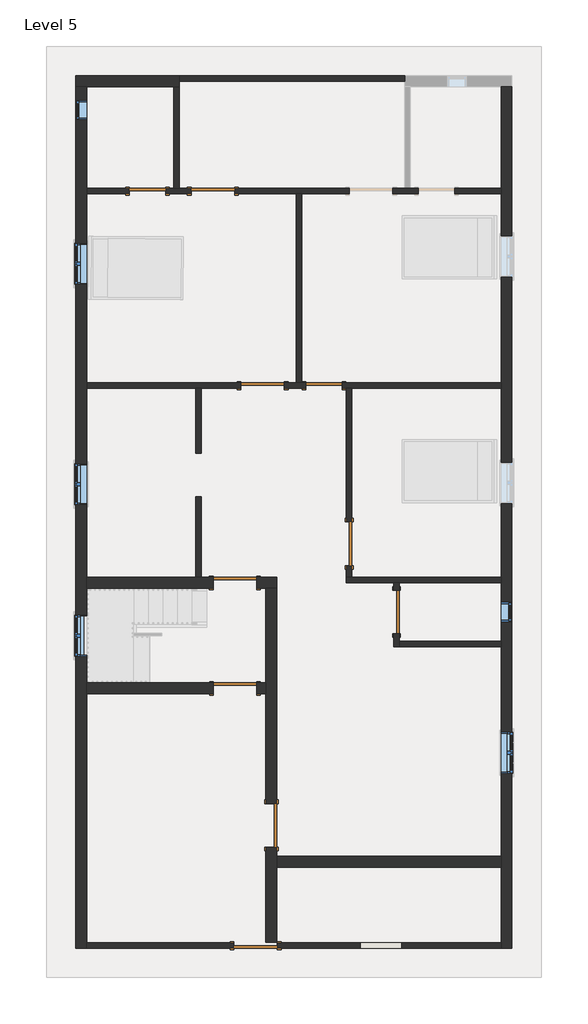
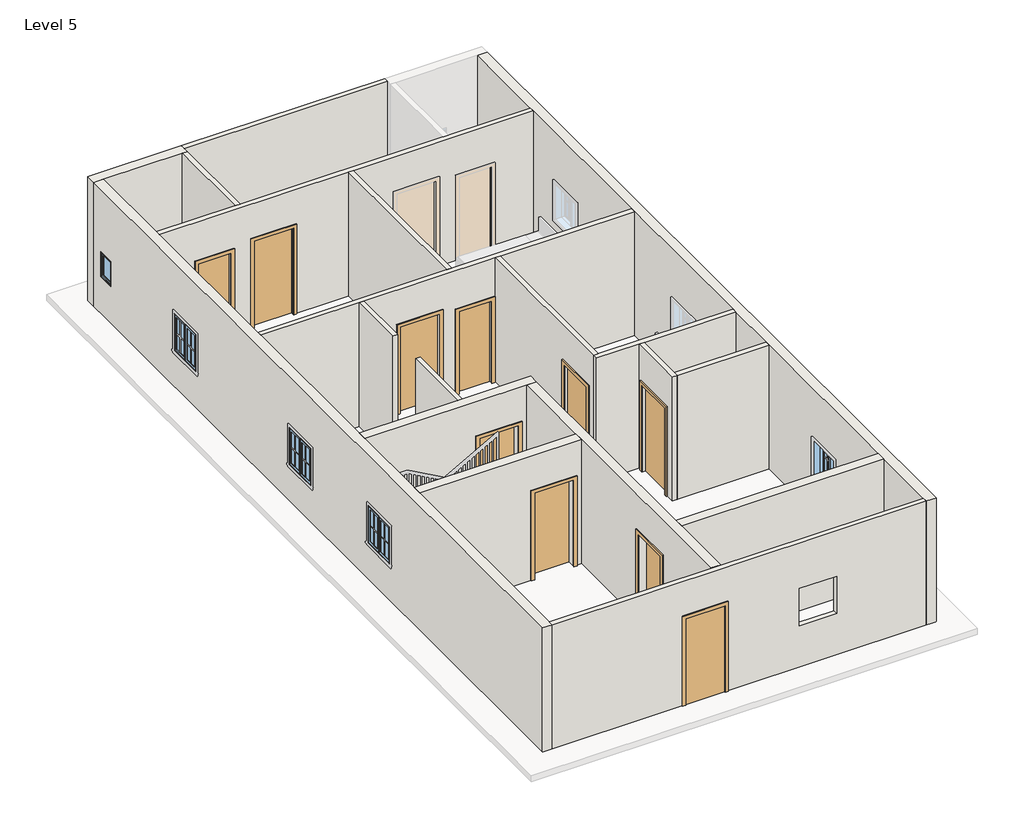
# One storey, part 1 of 3: 19 walls, 10 doors, 6 windows.
"""IFC4 building model written with IfcOpenShell, lengths in millimetres."""

from ifc_helpers import new_model, si_unit, frame, origin, place, context, project, spatial, polyline, outline, extrude, faceted_brep, transform, mapped, element, save
from components import door_d8f5dbb5, door_f2b275c1, door_e5f9f3c4, door_0ca8825f, door_305aa2a5, window_aa618e30, window_339605e1

model = new_model("IFC4")

# Units and contexts
model_context = context("Model", 3, world=origin())
ifc_project = project(units=[si_unit("LENGTHUNIT", "METRE", prefix="MILLI")], contexts=[model_context])

# Site, building, storey
site = spatial("IfcSite", under=ifc_project)
building = spatial("IfcBuilding", under=site)
storey = spatial("IfcBuildingStorey", under=building, Name="Level 5", Elevation=9601.2)

# Doors
placement = place(None, origin())
door_shape = door_d8f5dbb5(model_context)
element("IfcDoor", 1, ObjectType="Single-Flush : 30\" x 80\"", at=placement, inside=storey, context=model_context, shape_type="MappedRepresentation", body=[
    mapped(door_shape, transform((-4322.2915084, 8007.7072267, 9601.2), x_axis=(1.0, 0.0, 0.0), y_axis=(0.0, 1.0, 0.0), z_axis=(0.0, 0.0, 1.0))),
])
door_2_shape = door_f2b275c1(model_context)
element("IfcDoor", 2, ObjectType="Single-Flush : 30\" x 80\"", at=placement, inside=storey, context=model_context, shape_type="MappedRepresentation", body=[
    mapped(door_2_shape, transform((-621.124692, 3931.0072267, 9601.2), x_axis=(-1.0, 0.0, 0.0), y_axis=(0.0, -1.0, 0.0), z_axis=(0.0, 0.0, 1.0))),
])
door_3_shape = door_e5f9f3c4(model_context)
element("IfcDoor", 3, ObjectType="Single-Flush : 36\" x 84\"", at=placement, inside=storey, context=model_context, shape_type="MappedRepresentation", body=[
    mapped(door_3_shape, transform((-1909.2915084, 3931.0072267, 9601.2), x_axis=(1.0, 0.0, 0.0), y_axis=(0.0, 1.0, 0.0), z_axis=(0.0, 0.0, 1.0))),
])
element("IfcDoor", 4, ObjectType="Single-Flush : 36\" x 84\"", at=placement, inside=storey, context=model_context, shape_type="MappedRepresentation", body=[
    mapped(door_3_shape, transform((-94.9578757, 616.3072267, 9601.2), x_axis=(0.0, -1.0, 0.0), y_axis=(1.0, 0.0, 0.0), z_axis=(0.0, 0.0, 1.0))),
])
element("IfcDoor", 5, ObjectType="Single-Flush : 36\" x 84\"", at=placement, inside=storey, context=model_context, shape_type="MappedRepresentation", body=[
    mapped(door_3_shape, transform((-2055.3415084, -7803.7927733, 9601.2), x_axis=(-1.0, 0.0, 0.0), y_axis=(0.0, -1.0, 0.0), z_axis=(0.0, 0.0, 1.0))),
])
door_4_shape = door_0ca8825f(model_context)
element("IfcDoor", 6, ObjectType="Single-Flush : 36\" x 84\"", at=placement, inside=storey, context=model_context, shape_type="MappedRepresentation", body=[
    mapped(door_4_shape, transform((-2490.3165084, -202.8427733, 9601.2), x_axis=(1.0, 0.0, 0.0), y_axis=(0.0, 1.0, 0.0), z_axis=(0.0, 0.0, 1.0))),
])
element("IfcDoor", 7, ObjectType="Single-Flush : 36\" x 84\"", at=placement, inside=storey, context=model_context, shape_type="MappedRepresentation", body=[
    mapped(door_4_shape, transform((-2487.1415084, -2412.6427733, 9601.2), x_axis=(1.0, 0.0, 0.0), y_axis=(0.0, 1.0, 0.0), z_axis=(0.0, 0.0, 1.0))),
])
element("IfcDoor", 8, ObjectType="Single-Flush : 36\" x 84\"", at=placement, inside=storey, context=model_context, shape_type="MappedRepresentation", body=[
    mapped(door_4_shape, transform((-1725.1415084, -5282.8427733, 9601.2), x_axis=(0.0, -1.0, 0.0), y_axis=(1.0, 0.0, 0.0), z_axis=(0.0, 0.0, 1.0))),
])
door_5_shape = door_305aa2a5(model_context)
element("IfcDoor", 9, ObjectType="Single-Flush : 36\" x 84\"", at=placement, inside=storey, context=model_context, shape_type="MappedRepresentation", body=[
    mapped(door_5_shape, transform((897.4084916, -812.4427733, 9601.2), x_axis=(0.0, 1.0, 0.0), y_axis=(-1.0, 0.0, 0.0), z_axis=(0.0, 0.0, 1.0))),
])
element("IfcDoor", 10, ObjectType="Single-Flush : 36\" x 84\"", at=placement, inside=storey, context=model_context, shape_type="MappedRepresentation", body=[
    mapped(door_5_shape, transform((-2950.6915084, 8007.7072267, 9601.2), x_axis=(-1.0, 0.0, 0.0), y_axis=(0.0, -1.0, 0.0), z_axis=(0.0, 0.0, 1.0))),
])

# Walls
element("IfcWall", 11, ObjectType="WALL4.5\"", at=placement, inside=storey, context=model_context, shape_type="Brep", body=[
    faceted_brep([(821.2084916, 7950.5572267, 11734.8), (821.2084916, 7950.5572267, 9601.2), (1354.6084916, 7950.5572267, 9601.2), (1354.6084916, 7950.5572267, 11633.2), (2116.6084916, 7950.5572267, 11633.2), (2116.6084916, 7950.5572267, 9601.2), (3088.1584916, 7950.5572267, 9601.2), (3088.1584916, 7950.5572267, 12649.2), (-1090.1415084, 7950.5572267, 12649.2), (-1204.4415084, 7950.5572267, 12649.2), (-5598.6415084, 7950.5572267, 12649.2), (-5598.6415084, 7950.5572267, 9601.2), (-4703.2915084, 7950.5572267, 9601.2), (-4703.2915084, 7950.5572267, 11633.2), (-3941.2915084, 7950.5572267, 11633.2), (-3941.2915084, 7950.5572267, 9601.2), (-3407.8915084, 7950.5572267, 9601.2), (-3407.8915084, 7950.5572267, 11734.8), (-2493.4915084, 7950.5572267, 11734.8), (-2493.4915084, 7950.5572267, 9601.2), (-1204.4415084, 7950.5572267, 9601.2), (-1090.1415084, 7950.5572267, 9601.2), (-93.1915084, 7950.5572267, 9601.2), (-93.1915084, 7950.5572267, 11734.8), (1354.6084916, 8064.8572267, 9601.2), (1183.1584916, 8064.8572267, 9601.2), (1068.8584916, 8064.8572267, 9601.2), (821.2084916, 8064.8572267, 9601.2), (821.2084916, 8064.8572267, 11734.8), (-93.1915084, 8064.8572267, 11734.8), (-93.1915084, 8064.8572267, 9601.2), (-2493.4915084, 8064.8572267, 9601.2), (-2493.4915084, 8064.8572267, 11734.8), (-3407.8915084, 8064.8572267, 11734.8), (-3407.8915084, 8064.8572267, 9601.2), (-3655.5415084, 8064.8572267, 9601.2), (-3769.8415084, 8064.8572267, 9601.2), (-3941.2915084, 8064.8572267, 9601.2), (-3941.2915084, 8064.8572267, 11633.2), (-4703.2915084, 8064.8572267, 11633.2), (-4703.2915084, 8064.8572267, 9601.2), (-5598.6415084, 8064.8572267, 9601.2), (-5598.6415084, 8064.8572267, 12649.2), (-3769.8415084, 8064.8572267, 12649.2), (-3655.5415084, 8064.8572267, 12649.2), (1068.8584916, 8064.8572267, 12649.2), (1183.1584916, 8064.8572267, 12649.2), (3088.1584916, 8064.8572267, 12649.2), (3088.1584916, 8064.8572267, 9601.2), (2116.6084916, 8064.8572267, 9601.2), (2116.6084916, 8064.8572267, 11633.2), (1354.6084916, 8064.8572267, 11633.2)], [[[0, 1, 2, 3, 4, 5, 6, 7, 8, 9, 10, 11, 12, 13, 14, 15, 16, 17, 18, 19, 20, 21, 22, 23]], [[24, 25, 26, 27, 28, 29, 30, 31, 32, 33, 34, 35, 36, 37, 38, 39, 40, 41, 42, 43, 44, 45, 46, 47, 48, 49, 50, 51]], [[12, 11, 41, 40]], [[49, 48, 6, 5]], [[37, 36, 35, 34, 16, 15]], [[2, 1, 27, 26, 25, 24]], [[22, 21, 20, 19, 31, 30]], [[11, 10, 42, 41]], [[7, 6, 48, 47]], [[38, 37, 15, 14]], [[39, 38, 14, 13]], [[40, 39, 13, 12]], [[3, 2, 24, 51]], [[4, 3, 51, 50]], [[5, 4, 50, 49]], [[17, 16, 34, 33]], [[18, 17, 33, 32]], [[19, 18, 32, 31]], [[28, 27, 1, 0]], [[29, 28, 0, 23]], [[30, 29, 23, 22]], [[10, 9, 8, 7, 47, 46, 45, 44, 43, 42]]]),
])
element("IfcWall", 12, ObjectType="WALL4.5\"", at=placement, inside=storey, context=model_context, shape_type="SweptSolid", body=[
    extrude(outline(polyline([(-3769.8415084, 8064.8572267), (-3769.8415084, 10198.4572267), (-3655.5415084, 10198.4572267), (-3655.5415084, 8064.8572267), (-3769.8415084, 8064.8572267)])), frame((0.0, 0.0, 9601.2), z_axis=(0.0, 0.0, 1.0), x_axis=(1.0, 0.0, 0.0)), (0.0, 0.0, 1.0), 3048.0),
])
element("IfcWall", 13, ObjectType="WALL4.5\"", at=placement, inside=storey, context=model_context, shape_type="SweptSolid", body=[
    extrude(outline(polyline([(-1204.4415084, 3988.1572267), (-1204.4415084, 7950.5572267), (-1090.1415084, 7950.5572267), (-1090.1415084, 3988.1572267), (-1204.4415084, 3988.1572267)])), frame((0.0, 0.0, 9601.2), z_axis=(0.0, 0.0, 1.0), x_axis=(1.0, 0.0, 0.0)), (0.0, 0.0, 1.0), 3048.0),
])
element("IfcWall", 14, ObjectType="WALL4.5\"", at=placement, inside=storey, context=model_context, shape_type="Brep", body=[
    faceted_brep([(-1452.0915084, 3873.8572267, 9601.2), (-1002.124692, 3873.8572267, 9601.2), (-1002.124692, 3873.8572267, 11633.2), (-240.124692, 3873.8572267, 11633.2), (-240.124692, 3873.8572267, 9601.2), (-152.1078757, 3873.8572267, 9601.2), (-37.8078757, 3873.8572267, 9601.2), (3088.1584916, 3873.8572267, 9601.2), (3088.1584916, 3873.8572267, 12649.2), (-37.8078757, 3873.8572267, 12649.2), (-152.1078757, 3873.8572267, 12649.2), (-3198.3415084, 3873.8572267, 12649.2), (-3312.6415084, 3873.8572267, 12649.2), (-5598.6415084, 3873.8572267, 12649.2), (-5598.6415084, 3873.8572267, 9601.2), (-3312.6415084, 3873.8572267, 9601.2), (-3198.3415084, 3873.8572267, 9601.2), (-2366.4915084, 3873.8572267, 9601.2), (-2366.4915084, 3873.8572267, 11734.8), (-1452.0915084, 3873.8572267, 11734.8), (-1002.124692, 3988.1572267, 11633.2), (-1002.124692, 3988.1572267, 9601.2), (-1090.1415084, 3988.1572267, 9601.2), (-1204.4415084, 3988.1572267, 9601.2), (-1452.0915084, 3988.1572267, 9601.2), (-1452.0915084, 3988.1572267, 11734.8), (-2366.4915084, 3988.1572267, 11734.8), (-2366.4915084, 3988.1572267, 9601.2), (-5598.6415084, 3988.1572267, 9601.2), (-5598.6415084, 3988.1572267, 12649.2), (-1204.4415084, 3988.1572267, 12649.2), (-1090.1415084, 3988.1572267, 12649.2), (3088.1584916, 3988.1572267, 12649.2), (3088.1584916, 3988.1572267, 9601.2), (-240.124692, 3988.1572267, 9601.2), (-240.124692, 3988.1572267, 11633.2)], [[[0, 1, 2, 3, 4, 5, 6, 7, 8, 9, 10, 11, 12, 13, 14, 15, 16, 17, 18, 19]], [[20, 21, 22, 23, 24, 25, 26, 27, 28, 29, 30, 31, 32, 33, 34, 35]], [[17, 16, 15, 14, 28, 27]], [[34, 33, 7, 6, 5, 4]], [[24, 23, 22, 21, 1, 0]], [[14, 13, 29, 28]], [[8, 7, 33, 32]], [[25, 24, 0, 19]], [[26, 25, 19, 18]], [[27, 26, 18, 17]], [[2, 1, 21, 20]], [[3, 2, 20, 35]], [[4, 3, 35, 34]], [[13, 12, 11, 10, 9, 8, 32, 31, 30, 29]]]),
])
element("IfcWall", 15, ObjectType="WALL4.5\"", at=placement, inside=storey, context=model_context, shape_type="SweptSolid", body=[
    extrude(outline(polyline([(-3312.6415084, 2514.5843832), (-3312.6415084, 3873.8572267), (-3198.3415084, 3873.8572267), (-3198.3415084, 2514.5843832), (-3312.6415084, 2514.5843832)])), frame((0.0, 0.0, 9601.2), z_axis=(0.0, 0.0, 1.0), x_axis=(1.0, 0.0, 0.0)), (0.0, 0.0, 1.0), 3048.0),
])
element("IfcWall", 16, ObjectType="WALL4.5\"", at=placement, inside=storey, context=model_context, shape_type="SweptSolid", body=[
    extrude(outline(polyline([(-3312.6415084, -88.5427733), (-3312.6415084, 1600.2092553), (-3198.3415084, 1600.2092553), (-3198.3415084, -88.5427733), (-3312.6415084, -88.5427733)])), frame((0.0, 0.0, 9601.2), z_axis=(0.0, 0.0, 1.0), x_axis=(1.0, 0.0, 0.0)), (0.0, 0.0, 1.0), 3048.0),
])
element("IfcWall", 17, ObjectType="WALL4.5\"", at=placement, inside=storey, context=model_context, shape_type="SweptSolid", body=[
    extrude(outline(polyline([(159.1072267, 11734.8), (159.1072267, 9601.2), (-88.5427733, 9601.2), (-88.5427733, 12649.2), (3873.8572267, 12649.2), (3873.8572267, 9601.2), (1073.5072267, 9601.2), (1073.5072267, 11734.8), (159.1072267, 11734.8)])), frame((-152.1078757, 0.0, 0.0), z_axis=(1.0, 0.0, 0.0), x_axis=(0.0, 1.0, 0.0)), (0.0, 0.0, 1.0), 114.3),
])
element("IfcWall", 18, ObjectType="WALL4.5\"", at=placement, inside=storey, context=model_context, shape_type="Brep", body=[
    faceted_brep([(-152.1078757, -202.8427733, 9601.2), (840.2584916, -202.8427733, 9601.2), (954.5584916, -202.8427733, 9601.2), (3088.1584916, -202.8427733, 9601.2), (3088.1584916, -202.8427733, 12649.2), (954.5584916, -202.8427733, 12649.2), (840.2584916, -202.8427733, 12649.2), (-152.1078757, -202.8427733, 12649.2), (-152.1078757, -88.5427733, 9601.2), (-152.1078757, -88.5427733, 12649.2), (-37.8078757, -88.5427733, 12649.2), (3088.1584916, -88.5427733, 12649.2), (3088.1584916, -88.5427733, 9601.2), (-37.8078757, -88.5427733, 9601.2)], [[[0, 1, 2, 3, 4, 5, 6, 7]], [[8, 9, 10, 11, 12, 13]], [[3, 2, 1, 0, 8, 13, 12]], [[4, 3, 12, 11]], [[0, 7, 9, 8]], [[7, 6, 5, 4, 11, 10, 9]]]),
])
element("IfcWall", 19, ObjectType="WALL4.5\"", at=placement, inside=storey, context=model_context, shape_type="Brep", body=[
    faceted_brep([(840.2584916, -202.8427733, 9601.2), (840.2584916, -355.2427733, 9601.2), (840.2584916, -355.2427733, 11734.8), (840.2584916, -1269.6427733, 11734.8), (840.2584916, -1269.6427733, 9601.2), (840.2584916, -1536.3427733, 9601.2), (840.2584916, -1536.3427733, 12649.2), (840.2584916, -202.8427733, 12649.2), (954.5584916, -355.2427733, 11734.8), (954.5584916, -355.2427733, 9601.2), (954.5584916, -202.8427733, 9601.2), (954.5584916, -202.8427733, 12649.2), (954.5584916, -1422.0427733, 12649.2), (954.5584916, -1536.3427733, 12649.2), (954.5584916, -1536.3427733, 9601.2), (954.5584916, -1422.0427733, 9601.2), (954.5584916, -1269.6427733, 9601.2), (954.5584916, -1269.6427733, 11734.8)], [[[0, 1, 2, 3, 4, 5, 6, 7]], [[8, 9, 10, 11, 12, 13, 14, 15, 16, 17]], [[10, 9, 1, 0]], [[16, 15, 14, 5, 4]], [[0, 7, 11, 10]], [[6, 5, 14, 13]], [[2, 1, 9, 8]], [[3, 2, 8, 17]], [[4, 3, 17, 16]], [[7, 6, 13, 12, 11]]]),
])
element("IfcWall", 20, ObjectType="WALL4.5\"", at=placement, inside=storey, context=model_context, shape_type="SweptSolid", body=[
    extrude(outline(polyline([(3088.1584916, -1536.3427733), (954.5584916, -1536.3427733), (954.5584916, -1422.0427733), (3088.1584916, -1422.0427733), (3088.1584916, -1536.3427733)])), frame((0.0, 0.0, 9601.2), z_axis=(0.0, 0.0, 1.0), x_axis=(1.0, 0.0, 0.0)), (0.0, 0.0, 1.0), 3048.0),
])
element("IfcWall", 21, ObjectType="WALL4.5\"", at=placement, inside=storey, context=model_context, shape_type="SweptSolid", body=[
    extrude(outline(polyline([(9601.2, -5598.6415084), (9601.2, -2512.5415084), (11734.8, -2512.5415084), (11734.8, -1598.1415084), (9601.2, -1598.1415084), (9601.2, 3088.1584916), (12649.2, 3088.1584916), (12649.2, -5598.6415084), (9601.2, -5598.6415084)]), holes=[polyline([(11529.8022943, 141.7584916), (11529.8022943, 1005.3584916), (10615.4022943, 1005.3584916), (10615.4022943, 141.7584916), (11529.8022943, 141.7584916)])]), frame((0.0, -7860.9427733, 0.0), z_axis=(0.0, 1.0, 0.0), x_axis=(0.0, 0.0, 1.0)), (0.0, 0.0, 1.0), 114.3),
])
element("IfcWall", 22, ObjectType="WALL4.5\"", at=placement, inside=storey, context=model_context, shape_type="SweptSolid", body=[
    extrude(outline(polyline([(1068.8584916, 10312.7572267), (-3655.5415084, 10312.7572267), (-3655.5415084, 10427.0572267), (1068.8584916, 10427.0572267), (1068.8584916, 10312.7572267)])), frame((0.0, 0.0, 9601.2), z_axis=(0.0, 0.0, 1.0), x_axis=(1.0, 0.0, 0.0)), (0.0, 0.0, 1.0), 3048.0),
])
element("IfcWall", 23, ObjectType="WALL9\"", at=placement, inside=storey, context=model_context, shape_type="Brep", body=[
    faceted_brep([(-3655.5415084, 10427.0572267, 9601.2), (-5827.2415084, 10427.0572267, 9601.2), (-5827.2415084, 10427.0572267, 12649.2), (-3655.5415084, 10427.0572267, 12649.2), (-3655.5415084, 10198.4572267, 9601.2), (-3655.5415084, 10198.4572267, 12649.2), (-3769.8415084, 10198.4572267, 12649.2), (-5598.6415084, 10198.4572267, 12649.2), (-5827.2415084, 10198.4572267, 12649.2), (-5827.2415084, 10198.4572267, 9601.2), (-5598.6415084, 10198.4572267, 9601.2), (-3769.8415084, 10198.4572267, 9601.2), (-3655.5415084, 10312.7572267, 9601.2), (-3655.5415084, 10312.7572267, 12649.2)], [[[0, 1, 2, 3]], [[4, 5, 6, 7, 8, 9, 10, 11]], [[1, 0, 12, 4, 11, 10, 9]], [[2, 1, 9, 8]], [[0, 3, 13, 5, 4, 12]], [[3, 2, 8, 7, 6, 5, 13]]]),
])
element("IfcWall", 24, ObjectType="WALL9\"", at=placement, inside=storey, context=model_context, shape_type="Brep", body=[
    faceted_brep([(-5827.2415084, 10198.4572267, 9601.2), (-5827.2415084, -7860.9427733, 9601.2), (-5827.2415084, -7860.9427733, 12649.2), (-5827.2415084, 10198.4572267, 12649.2), (-5827.2415084, 9906.3572267, 11125.2), (-5827.2415084, 9499.9572267, 11125.2), (-5827.2415084, 9499.9572267, 10515.6), (-5827.2415084, 9906.3572267, 10515.6), (-5827.2415084, 6915.5072267, 11430.0), (-5827.2415084, 6051.9072267, 11430.0), (-5827.2415084, 6051.9072267, 10515.6), (-5827.2415084, 6915.5072267, 10515.6), (-5827.2415084, 2295.8822267, 11430.0), (-5827.2415084, 1432.2822267, 11430.0), (-5827.2415084, 1432.2822267, 10515.6), (-5827.2415084, 2295.8822267, 10515.6), (-5827.2415084, -875.9427733, 11430.0), (-5827.2415084, -1739.5427733, 11430.0), (-5827.2415084, -1739.5427733, 10515.6), (-5827.2415084, -875.9427733, 10515.6), (-5598.6415084, 10198.4572267, 9601.2), (-5598.6415084, 10198.4572267, 12649.2), (-5598.6415084, 8064.8572267, 12649.2), (-5598.6415084, 7950.5572267, 12649.2), (-5598.6415084, 3988.1572267, 12649.2), (-5598.6415084, 3873.8572267, 12649.2), (-5598.6415084, -88.5427733, 12649.2), (-5598.6415084, -317.1427733, 12649.2), (-5598.6415084, -2298.3427733, 12649.2), (-5598.6415084, -2526.9427733, 12649.2), (-5598.6415084, -7746.6427733, 12649.2), (-5598.6415084, -7860.9427733, 12649.2), (-5598.6415084, -7860.9427733, 9601.2), (-5598.6415084, -7746.6427733, 9601.2), (-5598.6415084, -2526.9427733, 9601.2), (-5598.6415084, -2298.3427733, 9601.2), (-5598.6415084, -317.1427733, 9601.2), (-5598.6415084, -88.5427733, 9601.2), (-5598.6415084, 3873.8572267, 9601.2), (-5598.6415084, 3988.1572267, 9601.2), (-5598.6415084, 7950.5572267, 9601.2), (-5598.6415084, 8064.8572267, 9601.2), (-5598.6415084, 9906.3572267, 11125.2), (-5598.6415084, 9906.3572267, 10515.6), (-5598.6415084, 9499.9572267, 10515.6), (-5598.6415084, 9499.9572267, 11125.2), (-5598.6415084, 6915.5072267, 11430.0), (-5598.6415084, 6915.5072267, 10515.6), (-5598.6415084, 6051.9072267, 10515.6), (-5598.6415084, 6051.9072267, 11430.0), (-5598.6415084, 2295.8822267, 11430.0), (-5598.6415084, 2295.8822267, 10515.6), (-5598.6415084, 1432.2822267, 10515.6), (-5598.6415084, 1432.2822267, 11430.0), (-5598.6415084, -875.9427733, 11430.0), (-5598.6415084, -875.9427733, 10515.6), (-5598.6415084, -1739.5427733, 10515.6), (-5598.6415084, -1739.5427733, 11430.0)], [[[0, 1, 2, 3], [4, 5, 6, 7], [8, 9, 10, 11], [12, 13, 14, 15], [16, 17, 18, 19]], [[20, 21, 22, 23, 24, 25, 26, 27, 28, 29, 30, 31, 32, 33, 34, 35, 36, 37, 38, 39, 40, 41], [42, 43, 44, 45], [46, 47, 48, 49], [50, 51, 52, 53], [54, 55, 56, 57]], [[1, 0, 20, 41, 40, 39, 38, 37, 36, 35, 34, 33, 32]], [[0, 3, 21, 20]], [[2, 1, 32, 31]], [[43, 42, 4, 7]], [[44, 43, 7, 6]], [[45, 44, 6, 5]], [[42, 45, 5, 4]], [[47, 46, 8, 11]], [[48, 47, 11, 10]], [[49, 48, 10, 9]], [[46, 49, 9, 8]], [[51, 50, 12, 15]], [[52, 51, 15, 14]], [[53, 52, 14, 13]], [[50, 53, 13, 12]], [[55, 54, 16, 19]], [[56, 55, 19, 18]], [[57, 56, 18, 17]], [[54, 57, 17, 16]], [[3, 2, 31, 30, 29, 28, 27, 26, 25, 24, 23, 22, 21]]]),
])
element("IfcWall", 25, ObjectType="WALL9\"", at=placement, inside=storey, context=model_context, shape_type="Brep", body=[
    faceted_brep([(3088.1584916, 10198.4572267, 9601.2), (3088.1584916, 8064.8572267, 9601.2), (3088.1584916, 7950.5572267, 9601.2), (3088.1584916, 3988.1572267, 9601.2), (3088.1584916, 3873.8572267, 9601.2), (3088.1584916, -88.5427733, 9601.2), (3088.1584916, -202.8427733, 9601.2), (3088.1584916, -1422.0427733, 9601.2), (3088.1584916, -1536.3427733, 9601.2), (3088.1584916, -5930.5427733, 9601.2), (3088.1584916, -6159.1427733, 9601.2), (3088.1584916, -7746.6427733, 9601.2), (3088.1584916, -7860.9427733, 9601.2), (3088.1584916, -7860.9427733, 12649.2), (3088.1584916, -7746.6427733, 12649.2), (3088.1584916, -6159.1427733, 12649.2), (3088.1584916, -5930.5427733, 12649.2), (3088.1584916, -1536.3427733, 12649.2), (3088.1584916, -1422.0427733, 12649.2), (3088.1584916, -202.8427733, 12649.2), (3088.1584916, -88.5427733, 12649.2), (3088.1584916, 3873.8572267, 12649.2), (3088.1584916, 3988.1572267, 12649.2), (3088.1584916, 7950.5572267, 12649.2), (3088.1584916, 8064.8572267, 12649.2), (3088.1584916, 10198.4572267, 12649.2), (3088.1584916, -1015.6427733, 11125.2), (3088.1584916, -1015.6427733, 10515.6), (3088.1584916, -609.2427733, 10515.6), (3088.1584916, -609.2427733, 11125.2), (3088.1584916, 6204.3072267, 11430.0), (3088.1584916, 6204.3072267, 10515.6), (3088.1584916, 7067.9072267, 10515.6), (3088.1584916, 7067.9072267, 11430.0), (3088.1584916, 1460.8572267, 11430.0), (3088.1584916, 1460.8572267, 10515.6), (3088.1584916, 2324.4572267, 10515.6), (3088.1584916, 2324.4572267, 11430.0), (3088.1584916, -4193.8177733, 11430.0), (3088.1584916, -4193.8177733, 10515.6), (3088.1584916, -3330.2177733, 10515.6), (3088.1584916, -3330.2177733, 11430.0), (3316.7584916, 10198.4572267, 9601.2), (3316.7584916, 10198.4572267, 12649.2), (3316.7584916, -7860.9427733, 12649.2), (3316.7584916, -7860.9427733, 9601.2), (3316.7584916, -1015.6427733, 11125.2), (3316.7584916, -609.2427733, 11125.2), (3316.7584916, -609.2427733, 10515.6), (3316.7584916, -1015.6427733, 10515.6), (3316.7584916, 6204.3072267, 11430.0), (3316.7584916, 7067.9072267, 11430.0), (3316.7584916, 7067.9072267, 10515.6), (3316.7584916, 6204.3072267, 10515.6), (3316.7584916, 1460.8572267, 11430.0), (3316.7584916, 2324.4572267, 11430.0), (3316.7584916, 2324.4572267, 10515.6), (3316.7584916, 1460.8572267, 10515.6), (3316.7584916, -4193.8177733, 11430.0), (3316.7584916, -3330.2177733, 11430.0), (3316.7584916, -3330.2177733, 10515.6), (3316.7584916, -4193.8177733, 10515.6)], [[[0, 1, 2, 3, 4, 5, 6, 7, 8, 9, 10, 11, 12, 13, 14, 15, 16, 17, 18, 19, 20, 21, 22, 23, 24, 25], [26, 27, 28, 29], [30, 31, 32, 33], [34, 35, 36, 37], [38, 39, 40, 41]], [[42, 43, 44, 45], [46, 47, 48, 49], [50, 51, 52, 53], [54, 55, 56, 57], [58, 59, 60, 61]], [[12, 11, 10, 9, 8, 7, 6, 5, 4, 3, 2, 1, 0, 42, 45]], [[0, 25, 43, 42]], [[13, 12, 45, 44]], [[27, 26, 46, 49]], [[28, 27, 49, 48]], [[29, 28, 48, 47]], [[26, 29, 47, 46]], [[31, 30, 50, 53]], [[32, 31, 53, 52]], [[33, 32, 52, 51]], [[30, 33, 51, 50]], [[35, 34, 54, 57]], [[36, 35, 57, 56]], [[37, 36, 56, 55]], [[34, 37, 55, 54]], [[39, 38, 58, 61]], [[40, 39, 61, 60]], [[41, 40, 60, 59]], [[38, 41, 59, 58]], [[25, 24, 23, 22, 21, 20, 19, 18, 17, 16, 15, 14, 13, 44, 43]]]),
])
element("IfcWall", 26, ObjectType="WALL9\"", at=placement, inside=storey, context=model_context, shape_type="Brep", body=[
    faceted_brep([(-2033.1165084, -317.1427733, 11734.8), (-2033.1165084, -317.1427733, 9601.2), (-1839.4415084, -317.1427733, 9601.2), (-1610.8415084, -317.1427733, 9601.2), (-1610.8415084, -317.1427733, 12649.2), (-1839.4415084, -317.1427733, 12649.2), (-5598.6415084, -317.1427733, 12649.2), (-5598.6415084, -317.1427733, 9601.2), (-2947.5165084, -317.1427733, 9601.2), (-2947.5165084, -317.1427733, 11734.8), (-1610.8415084, -88.5427733, 9601.2), (-2033.1165084, -88.5427733, 9601.2), (-2033.1165084, -88.5427733, 11734.8), (-2947.5165084, -88.5427733, 11734.8), (-2947.5165084, -88.5427733, 9601.2), (-3198.3415084, -88.5427733, 9601.2), (-3312.6415084, -88.5427733, 9601.2), (-5598.6415084, -88.5427733, 9601.2), (-5598.6415084, -88.5427733, 12649.2), (-3312.6415084, -88.5427733, 12649.2), (-3198.3415084, -88.5427733, 12649.2), (-1610.8415084, -88.5427733, 12649.2)], [[[0, 1, 2, 3, 4, 5, 6, 7, 8, 9]], [[10, 11, 12, 13, 14, 15, 16, 17, 18, 19, 20, 21]], [[8, 7, 17, 16, 15, 14]], [[3, 2, 1, 11, 10]], [[7, 6, 18, 17]], [[4, 3, 10, 21]], [[12, 11, 1, 0]], [[13, 12, 0, 9]], [[14, 13, 9, 8]], [[6, 5, 4, 21, 20, 19, 18]]]),
])
element("IfcWall", 27, ObjectType="WALL9\"", at=placement, inside=storey, context=model_context, shape_type="Brep", body=[
    faceted_brep([(-1839.4415084, -5740.0427733, 11734.8), (-1839.4415084, -5740.0427733, 9601.2), (-1839.4415084, -7733.9427733, 9601.2), (-1839.4415084, -7733.9427733, 12649.2), (-1839.4415084, -2526.9427733, 12649.2), (-1839.4415084, -2298.3427733, 12649.2), (-1839.4415084, -317.1427733, 12649.2), (-1839.4415084, -317.1427733, 9601.2), (-1839.4415084, -2298.3427733, 9601.2), (-1839.4415084, -2526.9427733, 9601.2), (-1839.4415084, -4825.6427733, 9601.2), (-1839.4415084, -4825.6427733, 11734.8), (-1610.8415084, -7733.9427733, 9601.2), (-1610.8415084, -6159.1427733, 9601.2), (-1610.8415084, -5930.5427733, 9601.2), (-1610.8415084, -5740.0427733, 9601.2), (-1610.8415084, -5740.0427733, 11734.8), (-1610.8415084, -4825.6427733, 11734.8), (-1610.8415084, -4825.6427733, 9601.2), (-1610.8415084, -317.1427733, 9601.2), (-1610.8415084, -317.1427733, 12649.2), (-1610.8415084, -5930.5427733, 12649.2), (-1610.8415084, -6159.1427733, 12649.2), (-1610.8415084, -7733.9427733, 12649.2)], [[[0, 1, 2, 3, 4, 5, 6, 7, 8, 9, 10, 11]], [[12, 13, 14, 15, 16, 17, 18, 19, 20, 21, 22, 23]], [[2, 1, 15, 14, 13, 12]], [[10, 9, 8, 7, 19, 18]], [[3, 2, 12, 23]], [[7, 6, 20, 19]], [[16, 15, 1, 0]], [[17, 16, 0, 11]], [[18, 17, 11, 10]], [[6, 5, 4, 3, 23, 22, 21, 20]]]),
])
element("IfcWall", 28, ObjectType="WALL9\"", at=placement, inside=storey, context=model_context, shape_type="SweptSolid", body=[
    extrude(outline(polyline([(3088.1584916, -6159.1427733), (-1610.8415084, -6159.1427733), (-1610.8415084, -5930.5427733), (3088.1584916, -5930.5427733), (3088.1584916, -6159.1427733)])), frame((0.0, 0.0, 9601.2), z_axis=(0.0, 0.0, 1.0), x_axis=(1.0, 0.0, 0.0)), (0.0, 0.0, 1.0), 3048.0),
])
element("IfcWall", 29, ObjectType="WALL9\"", at=placement, inside=storey, context=model_context, shape_type="SweptSolid", body=[
    extrude(outline(polyline([(11734.8, -2029.9415084), (9601.2, -2029.9415084), (9601.2, -1839.4415084), (12649.2, -1839.4415084), (12649.2, -5598.6415084), (9601.2, -5598.6415084), (9601.2, -2944.3415084), (11734.8, -2944.3415084), (11734.8, -2029.9415084)])), frame((0.0, -2526.9427733, 0.0), z_axis=(0.0, 1.0, 0.0), x_axis=(0.0, 0.0, 1.0)), (0.0, 0.0, 1.0), 228.6),
])

# Windows
window_shape = window_aa618e30(model_context)
element("IfcWindow", 30, ObjectType="Fixed : 16\" x 24\"", at=placement, inside=storey, context=model_context, shape_type="MappedRepresentation", body=[
    mapped(window_shape, transform((-5712.9415084, 9741.2572267, 9601.2), x_axis=(0.0, 1.0, 0.0), y_axis=(-1.0, 0.0, 0.0), z_axis=(0.0, 0.0, 1.0))),
])
element("IfcWindow", 31, ObjectType="Fixed : 16\" x 24\"", at=placement, inside=storey, context=model_context, shape_type="MappedRepresentation", body=[
    mapped(window_shape, transform((3202.4584916, -850.5427733, 9601.2), x_axis=(0.0, -1.0, 0.0), y_axis=(1.0, 0.0, 0.0), z_axis=(0.0, 0.0, 1.0))),
])
window_2_shape = window_339605e1(model_context)
element("IfcWindow", 32, ObjectType="Window-Casement-Double : 34\" x 36\"", at=placement, inside=storey, context=model_context, shape_type="MappedRepresentation", body=[
    mapped(window_2_shape, transform((-5712.9415084, 6483.7072267, 9601.2), x_axis=(0.0, 1.0, 0.0), y_axis=(-1.0, 0.0, 0.0), z_axis=(0.0, 0.0, 1.0))),
])
element("IfcWindow", 33, ObjectType="Window-Casement-Double : 34\" x 36\"", at=placement, inside=storey, context=model_context, shape_type="MappedRepresentation", body=[
    mapped(window_2_shape, transform((-5712.9415084, 1864.0822267, 9601.2), x_axis=(0.0, 1.0, 0.0), y_axis=(-1.0, 0.0, 0.0), z_axis=(0.0, 0.0, 1.0))),
])
element("IfcWindow", 34, ObjectType="Window-Casement-Double : 34\" x 36\"", at=placement, inside=storey, context=model_context, shape_type="MappedRepresentation", body=[
    mapped(window_2_shape, transform((3202.4584916, -3762.0177733, 9601.2), x_axis=(0.0, -1.0, 0.0), y_axis=(1.0, 0.0, 0.0), z_axis=(0.0, 0.0, 1.0))),
])
element("IfcWindow", 35, ObjectType="Window-Casement-Double : 34\" x 36\"", at=placement, inside=storey, context=model_context, shape_type="MappedRepresentation", body=[
    mapped(window_2_shape, transform((-5712.9415084, -1307.7427733, 9601.2), x_axis=(0.0, 1.0, 0.0), y_axis=(-1.0, 0.0, 0.0), z_axis=(0.0, 0.0, 1.0))),
])

save(model, "model.ifc")

# Revit data of these elements
# Type "Single-Flush : 30\" x 80\""
#   Type Mark = "5"
#   Construction Type Id = "MDOOR"
#   Assembly Code = "C1020"
#   Analytic Construction = "Metal"
#   Thickness = 0' - 2"
#   Heat Transfer Coefficient (U) = 0.651978 BTU/(h·ft²·°F)
#   Height = 6' - 8"
#   Trim Projection Ext = 0' - 1"
#   Trim Projection Int = 0' - 1"
#   Trim Width = 0' - 3"
#   Width = 2' - 6"
#   Define Thermal Properties by = 1
#   Define Thermal Properties by = 1
#   Door Material = Door - Panel
#   Frame Material = Door - Frame
#   Visual Light Transmittance = 0
#   Solar Heat Gain Coefficient = 0
#   Function = (empty or 0)
#   Wall Closure = (empty or 0)
# Type "Single-Flush : 36\" x 84\""
#   Type Mark = "1"
#   Construction Type Id = "MDOOR"
#   Assembly Code = "C1020"
#   Analytic Construction = "Metal"
#   Thickness = 0' - 2"
#   Heat Transfer Coefficient (U) = 0.651978 BTU/(h·ft²·°F)
#   Height = 7' - 0"
#   Trim Projection Ext = 0' - 1"
#   Trim Projection Int = 0' - 1"
#   Trim Width = 0' - 3"
#   Width = 3' - 0"
#   Define Thermal Properties by = 1
#   Define Thermal Properties by = 1
#   Door Material = Door - Panel
#   Frame Material = Door - Frame
#   Visual Light Transmittance = 0
#   Solar Heat Gain Coefficient = 0
#   Function = (empty or 0)
#   Wall Closure = (empty or 0)
# Type "WALL4.5\""
#   Assembly Code = "B2010"
#   Layers, outside or top first: 0' - 4 1/2" no material (function 1)
# Type "WALL9\""
#   Assembly Code = "B2010"
#   Layers, outside or top first: 0' - 9" no material (function 1)
# Type "Fixed : 16\" x 24\""
#   Type Mark = "4"
#   Construction Type Id = "GSP4R"
#   Assembly Code = "B2020100"
#   Analytic Construction = "1/8 in Pilkington single glazing"
#   Visual Light Transmittance = 0.9
#   Solar Heat Gain Coefficient = 0.78
#   Heat Transfer Coefficient (U) = 0.6496 BTU/(h·ft²·°F)
#   Height = 2' - 0"
#   Default Sill Height = 3' - 0"
#   Width = 1' - 4"
#   Window Inset = 0' - 0 3/4"
#   Define Thermal Properties by = 1
#   Define Thermal Properties by = 1
#   Glass Pane Material = Glass
#   Sash Material = Sash
#   Wall Closure = (empty or 0)
# Type "Window-Casement-Double : 34\" x 36\""
#   Type Mark = "14"
#   Fire Rating = "0.5h"
#   Assembly Code = "B2020100"
#   Analytic Construction = "Double glazing - domestic"
#   Frame Extension [instance default] = 0' - 0 1/4"
#   Window Inset [instance default] = 0' - 0"
#   Wall Thickness [instance default] = 0' - 6"
#   Interior Wall Closure [instance default] = 0' - 2 1/4"
#   Half Width = 1' - 5"
#   Visual Light Transmittance = 0.81
#   Thermal Resistance (R) = 1.8146 (h·ft²·°F)/BTU
#   Solar Heat Gain Coefficient = 0.76
#   Rough Width = 2' - 10 1/2"
#   Rough Height = 3' - 0 1/2"
#   Height = 3' - 0"
#   Heat Transfer Coefficient (U) = 0.5511 BTU/(h·ft²·°F)
#   Exterior Wall Closure [instance default] = 0' - 1 1/4"
#   Extension Jamb [instance default] = 0' - 2 1/4"
#   Default Sill Height = 3' - 0"
#   Width = 2' - 10"
#   Define Thermal Properties by = 0
#   Muntin Visibility = yes
#   Interior Trim Visibility [instance default] = yes
#   Exterior Trim Visibility [instance default] = yes
#   Extension Jamb Visibility [instance default] = yes
#   Interior Trim Material = Wood - Stained
#   Muntin Pattern = Muntin Pattern_2x2 : Muntin Pattern_2x2
#   Interior Trim = Trim-Window-Interior-Flat : Picture Frame
#   Interior Frame Material = Wood - Stained
#   Glass Panel Material = Glass
#   Exterior Trim Material = Clad - White
#   Exterior Trim = Trim-Window-Exterior-Flat : with Sill
#   Exterior Frame Material = Clad - White
#   Wall Closure = (empty or 0)
# Elements 1, 2 (IfcDoor, "Single-Flush : 30\" x 80\"")
#   Phase Created = New Construction
#   Materials on its faces: "Door - Frame", "Door - Panel"
# Elements 3, 4, 5, 6, 7, 8, 9, 10 (IfcDoor, "Single-Flush : 36\" x 84\"")
#   Phase Created = New Construction
#   Materials on its faces: "Door - Frame", "Door - Panel"
# Elements 11, 21, 22 (IfcWall, "WALL4.5\"")
#   Top Offset = 0' - 0"
#   Base Offset = 0' - 0"
#   Unconnected Height = 10' - 0"
#   wall height = 10' - 0"
#   Phase Created = New Construction
#   Base Constraint = Level 5
#   Materials on its faces: "Default Wall", "Wood Planks"
# Elements 12, 13, 14, 15, 16, 17, 18, 19, 20 (IfcWall, "WALL4.5\"")
#   Top Offset = 0' - 0"
#   Base Offset = 0' - 0"
#   Unconnected Height = 10' - 0"
#   wall height = 10' - 0"
#   Phase Created = New Construction
#   Base Constraint = Level 5
#   Materials on its faces: "Default Wall"
# Elements 23, 24, 25 (IfcWall, "WALL9\"")
#   Top Offset = 0' - 0"
#   Base Offset = 0' - 0"
#   Unconnected Height = 10' - 0"
#   wall height = 10' - 0"
#   Phase Created = New Construction
#   Base Constraint = Level 5
#   Materials on its faces: "Default Wall", "Wood Planks"
# Elements 26, 27, 28, 29 (IfcWall, "WALL9\"")
#   Top Offset = 0' - 0"
#   Base Offset = 0' - 0"
#   Unconnected Height = 10' - 0"
#   wall height = 10' - 0"
#   Phase Created = New Construction
#   Base Constraint = Level 5
#   Materials on its faces: "Default Wall"
# Element 30 (IfcWindow, "Fixed : 16\" x 24\"")
#   Mark = "28"
#   Phase Created = New Construction
#   Materials on its faces: "Sash", "Glass"
# Element 31 (IfcWindow, "Fixed : 16\" x 24\"")
#   Mark = "30"
#   Phase Created = New Construction
#   Materials on its faces: "Sash", "Glass"
# Element 32 (IfcWindow, "Window-Casement-Double : 34\" x 36\"")
#   Mark = "33"
#   Window Inset = 0' - 0"
#   Interior Wall Closure = 0' - 2 1/4"
#   Frame Extension = 0' - 0 1/4"
#   Exterior Wall Closure = 0' - 1 1/4"
#   Interior Trim Visibility = yes
#   Exterior Trim Visibility = yes
#   Phase Created = New Construction
#   Materials on its faces: "Wood - Stained", "Glass", "Clad - White"
# Element 33 (IfcWindow, "Window-Casement-Double : 34\" x 36\"")
#   Mark = "34"
#   Window Inset = 0' - 0"
#   Interior Wall Closure = 0' - 2 1/4"
#   Frame Extension = 0' - 0 1/4"
#   Exterior Wall Closure = 0' - 1 1/4"
#   Interior Trim Visibility = yes
#   Exterior Trim Visibility = yes
#   Phase Created = New Construction
#   Materials on its faces: "Wood - Stained", "Glass", "Clad - White"
# Element 34 (IfcWindow, "Window-Casement-Double : 34\" x 36\"")
#   Mark = "35"
#   Window Inset = 0' - 0"
#   Interior Wall Closure = 0' - 2 1/4"
#   Frame Extension = 0' - 0 1/4"
#   Exterior Wall Closure = 0' - 1 1/4"
#   Interior Trim Visibility = yes
#   Exterior Trim Visibility = yes
#   Phase Created = New Construction
#   Materials on its faces: "Wood - Stained", "Glass", "Clad - White"
# Element 35 (IfcWindow, "Window-Casement-Double : 34\" x 36\"")
#   Mark = "36"
#   Window Inset = 0' - 0"
#   Interior Wall Closure = 0' - 2 1/4"
#   Frame Extension = 0' - 0 1/4"
#   Exterior Wall Closure = 0' - 1 1/4"
#   Interior Trim Visibility = yes
#   Exterior Trim Visibility = yes
#   Phase Created = New Construction
#   Materials on its faces: "Wood - Stained", "Glass", "Clad - White"
# Materials
#   "Door - Panel": class "Wood", colour RGB 210 159 95, transparency 0, Cost = 0
#   "Door - Frame": colour RGB 118 70 51, transparency 0, Cost = 0
#   "Glass": class "Glass", colour RGB 0 128 192, transparency 0.75, Description = "Soda Lime Glass", Cost = 0
#   "Sash": class "Wood", colour RGB 224 178 126, transparency 0, Cost = 0
#   "Wood - Stained": class "Wood", colour RGB 224 178 126, transparency 0, Cost = 0
#   "Clad - White": class "Wood", colour RGB 242 242 238, transparency 0, Cost = 0
#   "Default Wall": colour RGB 128 128 128, transparency 0, Cost = 0
#   "Wood Planks": class "Wood", colour RGB 193 160 115, transparency 0, Description = "Physical material.", Cost = 0
